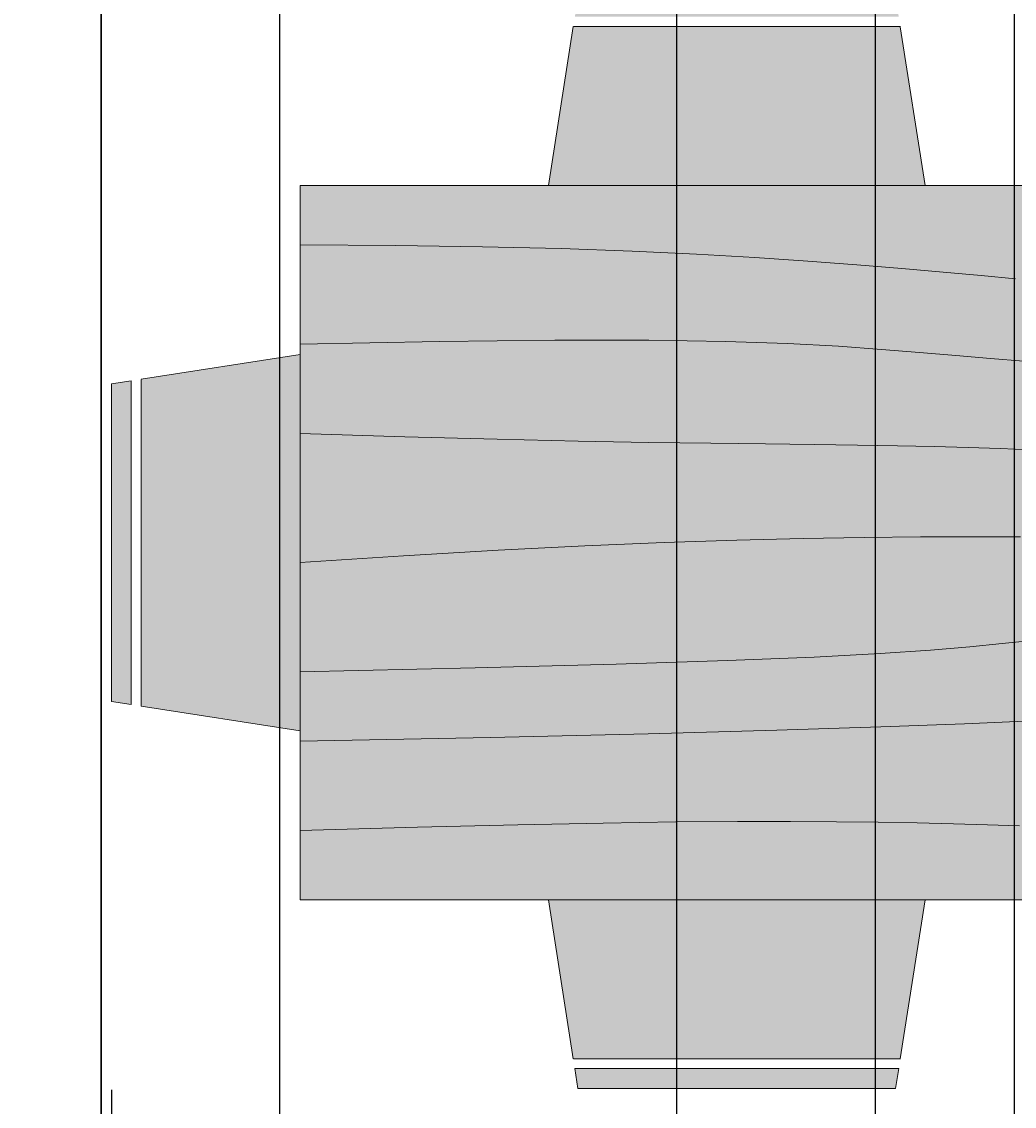
# Model space of a CAD drawing. Units: inches. Extents: x 1567 to 1964, y 1813 to 2447.
# Tile 17 of 28: x 1738 to 1788, y 2172 to 2226. Entities that reach past the tile are written whole.
import ezdxf

# ---------------------------------------------------------------- set-up
doc = ezdxf.new("R2010")
doc.units = ezdxf.units.IN
doc.layers.add('A-ANNO-DIMS', color=2, linetype='Continuous', lineweight=18)
doc.layers.add('A-FURN', color=8, linetype='Continuous', lineweight=18)
doc.layers.add('A-FURN-PATT', color=252, linetype='Continuous', lineweight=13, true_color=0x939598)
doc.styles.get("Standard").update_dxf_attribs({"font": 'arial.ttf'})
doc.dimstyles.get("Standard").update_dxf_attribs({"dimtxt": 0.18, "dimasz": 0.18, "dimexe": 0.18, "dimexo": 0.0625, "dimgap": 0.09, "dimtad": 0, "dimtih": 1, "dimtoh": 1, "dimdec": 4, "dimzin": 0, "dimdsep": 46, "dimtxsty": 'Standard', "dimcen": 0.09, "dimadec": 0, "dimazin": 0, "dimtfac": 1, "dimtdec": 4, "dimtofl": 0, "dimtmove": 0, "dimatfit": 3, "dimfxl": 1, "dimtolj": 1, "dimtzin": 0, "dimarcsym": 0})

# ---------------------------------------------------------------- blocks, each defined once
blk = doc.blocks.new('Dining Set - 36 x 72 in.')
for p, q in [((-22.2343, 26.00059), (-23.4847, 17.99762)), ((-22.2304, 26), (-5.7608, 26)), ((-4.5152, 17.99762), (-5.7655, 25.99926)), ((36, 18), (-36, 18)), ((-36, 18), (-36, -18)), ((-44.0006, 8.23428), (-35.9976, 9.48474)), ((-44, 8.23041), (-44, -8.23915)), ((-45.5, 8), (-44.5004, 8.15617)), ((-45.5, 8), (-45.5, -8)), ((-44.5, -8.15843), (-44.5, 8.15338)), ((-44.4997, -8.15631), (-45.5, -8)), ((-35.9976, -9.48476), (-43.9993, -8.2345)), ((-36, -18), (36, -18)), ((-22.2343, -26.0006), (-23.4847, -17.99762)), ((-4.5152, -17.99762), (-5.7655, -25.99928)), ((-22.2304, -26), (-5.7608, -26)), ((-22, -27.5), (-22.1562, -26.50044)), ((-5.8416, -26.5), (-22.1534, -26.5)), ((-5.8437, -26.49967), (-6, -27.5)), ((-22, -27.5), (-6, -27.5))]:
    blk.add_line(p, q)
for points in [[(-36, 15), (-31.1772, 14.97754), (-26.8079, 14.91406), (-22.8538, 14.81543), (-19.276, 14.6875), (-16.0362, 14.53613), (-13.0957, 14.36718), (-10.4159, 14.18652), (-7.9583, 14), (-5.6904, 13.81315), (-3.6035, 13.63021), (-1.6954, 13.45508), (0.0365, 13.29166)], [(-36, 10), (-28.9766, 10.14274), (-23.1725, 10.20442), (-18.4241, 10.19775), (-14.5677, 10.13541), (-11.4399, 10.03011), (-8.877, 9.89453), (-6.7154, 9.74137), (-4.7917, 9.58333), (-2.9698, 9.43082), (-1.2246, 9.28515), (0.4415, 9.14534)], [(-36, 5.5), (-30.7157, 5.3348), (-26.069, 5.20963), (-21.9946, 5.11767), (-18.4271, 5.05208), (-15.3009, 5.00602), (-12.5508, 4.97265), (-10.1112, 4.94515), (-7.9167, 4.91666), (-5.909, 4.88167), (-4.0586, 4.83984), (-2.3429, 4.79215), (-0.7396, 4.73958), (0.7739, 4.6831)], [(-36, -1), (-30.7915, -0.6591), (-26.0195, -0.38216), (-21.6519, -0.16284), (-17.6563, 0.00521), (-14.0005, 0.12833), (-10.6523, 0.21289), (-7.5796, 0.26522), (-4.75, 0.29166), (-2.134, 0.29793), (0.2878, 0.28711)], [(-36, -6.5), (-27.1843, -6.31267), (-20.084, -6.1263), (-14.469, -5.9419), (-10.1094, -5.76042), (-6.7752, -5.58285), (-4.2363, -5.41016), (-2.2629, -5.24333), (-0.625, -5.08334), (0.8708, -4.93099)], [(-36, -10), (-26.4022, -9.81299), (-18.4675, -9.62891), (-11.9839, -9.45069), (-6.7396, -9.28125), (-2.5226, -9.12354), (0.8789, -8.98047)], [(-36, -14.5), (-30.0881, -14.33513), (-25.0332, -14.21224), (-20.7312, -14.12647), (-17.0781, -14.07292), (-13.97, -14.04671), (-11.3027, -14.04297), (-8.9724, -14.05681), (-6.875, -14.08334), (-4.9224, -14.11833), (-3.0905, -14.16016), (-1.3709, -14.20785), (0.2448, -14.26042)]]:
    blk.add_lwpolyline(points)
blk = doc.blocks.new('*D27')
at = {"layer": 'A-ANNO-DIMS', "color": 0, "lineweight": -2, "transparency": 16777216}
for p, q in [((1742.951, 2172.357), (1742.951, 2158.59)), ((1833.951, 2172.357), (1833.951, 2158.59)), ((1743.131, 2158.77), (1787.5, 2158.77)), ((1833.771, 2158.77), (1789.403, 2158.77))]:
    blk.add_line(p, q, dxfattribs=at)
at = {"layer": 'A-ANNO-DIMS', "color": 0, "transparency": 16777216}
for points in [[(1743.131, 2158.8), (1743.131, 2158.74), (1742.951, 2158.77)], [(1833.771, 2158.8), (1833.771, 2158.74), (1833.951, 2158.77)]]:
    blk.add_solid(points, dxfattribs=at)
at = {"layer": 'Defpoints', "color": 0, "transparency": 16777216}
for p in [(1742.951, 2172.42), (1833.951, 2172.42), (1833.951, 2158.77)]:
    blk.add_point(p, dxfattribs=at)
at = {"layer": 'A-ANNO-DIMS', "color": 0, "transparency": 16777216, "insert": (1788.451, 2158.77), "char_height": 0.18, "attachment_point": 5}
blk.add_mtext('\\A1;DINING SET 91', dxfattribs=at)
blk = doc.blocks.new('*D47')
at = {"layer": 'A-ANNO-DIMS', "color": 0, "lineweight": -2, "transparency": 16777216}
for p, q in [((1742.43, 2331.227), (1742.43, 1813.46)), ((1788.43, 2331.227), (1788.43, 1813.46)), ((1742.61, 1813.64), (1765.207, 1813.64)), ((1788.25, 1813.64), (1765.652, 1813.64))]:
    blk.add_line(p, q, dxfattribs=at)
at = {"layer": 'A-ANNO-DIMS', "color": 0, "transparency": 16777216}
for points in [[(1742.61, 1813.67), (1742.61, 1813.61), (1742.43, 1813.64)], [(1788.25, 1813.67), (1788.25, 1813.61), (1788.43, 1813.64)]]:
    blk.add_solid(points, dxfattribs=at)
at = {"layer": 'Defpoints', "color": 0, "transparency": 16777216}
for p in [(1742.43, 2331.29), (1788.43, 2331.29), (1788.43, 1813.64)]:
    blk.add_point(p, dxfattribs=at)
at = {"layer": 'A-ANNO-DIMS', "color": 0, "transparency": 16777216, "insert": (1765.43, 1813.64), "char_height": 0.18, "attachment_point": 5}
blk.add_mtext('\\A1;46', dxfattribs=at)
blk = doc.blocks.new('*D54')
at = {"layer": 'A-ANNO-DIMS', "color": 0, "lineweight": -2, "transparency": 16777216}
for p, q in [((1711.43, 1964.352), (1711.43, 2447.12)), ((1711.61, 2446.94), (1753.211, 2446.94)), ((1795.25, 2446.94), (1753.648, 2446.94)), ((1795.43, 1964.352), (1795.43, 2447.12))]:
    blk.add_line(p, q, dxfattribs=at)
at = {"layer": 'A-ANNO-DIMS', "color": 0, "transparency": 16777216}
for points in [[(1711.61, 2446.97), (1711.61, 2446.91), (1711.43, 2446.94)], [(1795.25, 2446.97), (1795.25, 2446.91), (1795.43, 2446.94)]]:
    blk.add_solid(points, dxfattribs=at)
at = {"layer": 'Defpoints', "color": 0, "transparency": 16777216}
for p in [(1795.43, 2446.94), (1711.43, 1964.29), (1795.43, 1964.29)]:
    blk.add_point(p, dxfattribs=at)
at = {"layer": 'A-ANNO-DIMS', "color": 0, "transparency": 16777216, "insert": (1753.43, 2446.94), "char_height": 0.18, "attachment_point": 5}
blk.add_mtext('\\A1;84', dxfattribs=at)
blk = doc.blocks.new('*D58')
at = {"layer": 'A-ANNO-DIMS', "color": 0, "lineweight": -2, "transparency": 16777216}
for p, q in [((1742.43, 2127.352), (1742.43, 2447.12)), ((1742.61, 2446.94), (1746.78, 2446.94)), ((1751.25, 2446.94), (1747.079, 2446.94)), ((1751.43, 2127.352), (1751.43, 2447.12))]:
    blk.add_line(p, q, dxfattribs=at)
at = {"layer": 'A-ANNO-DIMS', "color": 0, "transparency": 16777216}
for points in [[(1742.61, 2446.97), (1742.61, 2446.91), (1742.43, 2446.94)], [(1751.25, 2446.97), (1751.25, 2446.91), (1751.43, 2446.94)]]:
    blk.add_solid(points, dxfattribs=at)
at = {"layer": 'Defpoints', "color": 0, "transparency": 16777216}
for p in [(1751.43, 2446.94), (1742.43, 2127.29), (1751.43, 2127.29)]:
    blk.add_point(p, dxfattribs=at)
at = {"layer": 'A-ANNO-DIMS', "color": 0, "transparency": 16777216, "insert": (1746.93, 2446.94), "char_height": 0.18, "attachment_point": 5}
blk.add_mtext('\\A1;9', dxfattribs=at)
blk = doc.blocks.new('*D59')
at = {"layer": 'A-ANNO-DIMS', "color": 0, "lineweight": -2, "transparency": 16777216}
for p, q in [((1751.43, 2127.352), (1751.43, 2447.12)), ((1751.61, 2446.94), (1766.211, 2446.94)), ((1781.25, 2446.94), (1766.648, 2446.94)), ((1781.43, 2127.352), (1781.43, 2447.12))]:
    blk.add_line(p, q, dxfattribs=at)
at = {"layer": 'A-ANNO-DIMS', "color": 0, "transparency": 16777216}
for points in [[(1751.61, 2446.97), (1751.61, 2446.91), (1751.43, 2446.94)], [(1781.25, 2446.97), (1781.25, 2446.91), (1781.43, 2446.94)]]:
    blk.add_solid(points, dxfattribs=at)
at = {"layer": 'Defpoints', "color": 0, "transparency": 16777216}
for p in [(1781.43, 2446.94), (1751.43, 2127.29), (1781.43, 2127.29)]:
    blk.add_point(p, dxfattribs=at)
at = {"layer": 'A-ANNO-DIMS', "color": 0, "transparency": 16777216, "insert": (1766.43, 2446.94), "char_height": 0.18, "attachment_point": 5}
blk.add_mtext('\\A1;30', dxfattribs=at)
blk = doc.blocks.new('*D63')
at = {"layer": 'A-ANNO-DIMS', "color": 0, "lineweight": -2, "transparency": 16777216}
for p, q in [((1735.43, 1988.352), (1735.43, 2447.12)), ((1735.61, 2446.94), (1753.211, 2446.94)), ((1771.25, 2446.94), (1753.648, 2446.94)), ((1771.43, 1988.352), (1771.43, 2447.12))]:
    blk.add_line(p, q, dxfattribs=at)
at = {"layer": 'A-ANNO-DIMS', "color": 0, "transparency": 16777216}
for points in [[(1735.61, 2446.97), (1735.61, 2446.91), (1735.43, 2446.94)], [(1771.25, 2446.97), (1771.25, 2446.91), (1771.43, 2446.94)]]:
    blk.add_solid(points, dxfattribs=at)
at = {"layer": 'Defpoints', "color": 0, "transparency": 16777216}
for p in [(1771.43, 2446.94), (1735.43, 1988.29), (1771.43, 1988.29)]:
    blk.add_point(p, dxfattribs=at)
at = {"layer": 'A-ANNO-DIMS', "color": 0, "transparency": 16777216, "insert": (1753.43, 2446.94), "char_height": 0.18, "attachment_point": 5}
blk.add_mtext('\\A1;36', dxfattribs=at)

msp = doc.modelspace()

# ---------------------------------------------------------------- hatches: boundary and pattern name
at = {"layer": 'A-FURN-PATT'}
h = msp.add_hatch(color=256, dxfattribs=at)
h.dxf.hatch_style = 1
h.paths.add_polyline_path([(1621.2532, 2242.0229), (1643.7811, 2241.7239), (1643.8607, 2247.7234), (1617.863, 2248.0685, 0.1904762), (1616.7481, 2164.0759), (1642.7458, 2163.7308), (1642.8254, 2169.7302), (1620.2975, 2170.0293, -0.1519478)])
h.paths.add_polyline_path([(1673.5306, 2249.6607), (1653.8509, 2249.6607), (1653.8509, 2248.5031, 0.1176471), (1673.5306, 2248.5031)])
h.paths.add_polyline_path([(1706.0889, 2249.6607), (1686.4092, 2249.6607), (1686.4092, 2248.5031, 0.1176471), (1706.0889, 2248.5031)])
h.paths.add_polyline_path([(1782.4511, 2227.4197), (1766.4511, 2227.4197), (1766.2949, 2226.4197), (1782.6074, 2226.4197)])
h.paths.add_polyline_path([(1810.4511, 2227.4197), (1794.4511, 2227.4197), (1794.2949, 2226.4197), (1810.6074, 2226.4197)])
h.paths.add_polyline_path([(1743.9511, 2208.076), (1742.9511, 2207.9197), (1742.9511, 2191.9197), (1743.9511, 2191.7635)])
h.paths.add_polyline_path([(1782.6074, 2173.4197), (1766.2949, 2173.4197), (1766.4511, 2172.4197), (1782.4511, 2172.4197)])
h.paths.add_polyline_path([(1810.6074, 2173.4197), (1794.2949, 2173.4197), (1794.4511, 2172.4197), (1810.4511, 2172.4197)])
h.paths.add_polyline_path([(1861.053, 2006.5071), (1845.8531, 2006.5071), (1861.053, 1991.3071)])
h.paths.add_polyline_path([(1905.853, 1993.7071), (1861.053, 1993.7071), (1861.053, 1991.3071), (1905.853, 1991.3071)])
h.paths.add_polyline_path([(1919.7245, 2257.29, 0.5000001), (1918.7245, 2258.29), (1901.7245, 2258.29, 0.5000001), (1900.7245, 2257.29), (1900.7245, 2253.29, 0.5000001), (1901.7245, 2252.29), (1918.7245, 2252.29, 0.5000001), (1919.7245, 2253.29)])
h.paths.add_polyline_path([(1875.9094, 2391.0204), (1875.9094, 2375.8204), (1891.1093, 2375.8204)], flags=17)
h.paths.add_polyline_path([(1891.1093, 2405.4204), (1831.1094, 2405.4204), (1831.1094, 2391.0204), (1839.1093, 2391.0204), (1839.1093, 2404.2204), (1859.9093, 2404.2204), (1859.9093, 2391.0204), (1862.3093, 2391.0204), (1862.3093, 2404.2204), (1883.1093, 2404.2204), (1883.1093, 2389.0204), (1877.9094, 2389.0204), (1891.1093, 2375.8204)])
h.paths.add_polyline_path([(1682.1402, 2390.0316), (1682.1402, 2374.8316), (1697.3402, 2374.8316)], flags=17)
h.paths.add_polyline_path([(1697.3402, 2404.4316), (1637.3402, 2404.4316), (1637.3402, 2390.0316), (1645.3402, 2390.0316), (1645.3402, 2403.2316), (1666.1402, 2403.2316), (1666.1402, 2390.0316), (1668.5402, 2390.0316), (1668.5402, 2403.2316), (1689.3402, 2403.2316), (1689.3402, 2388.0316), (1684.1402, 2388.0316), (1697.3402, 2374.8316)])
h = msp.add_hatch(color=256, dxfattribs=at)
h.dxf.hatch_style = 1
h.paths.add_polyline_path([(1697.3402, 2374.8316), (1682.1402, 2374.8316), (1682.1402, 2387.6316), (1637.3402, 2387.6316), (1637.3402, 2324.4315), (1697.3402, 2324.4315)])
h.paths.add_polyline_path([(1891.1093, 2375.8204), (1875.9094, 2375.8204), (1875.9094, 2388.6204), (1831.1094, 2388.6204), (1831.1094, 2325.4204), (1891.1093, 2325.4204)])
h.paths.add_polyline_path([(1702.5611, 2206.8057), (1702.5611, 2210.8057), (1699.7395, 2209.9436), (1697.013, 2209.2403), (1694.3857, 2208.6763), (1691.8615, 2208.2326), (1689.4443, 2207.8896), (1687.1381, 2207.6282), (1684.9469, 2207.4289), (1682.8747, 2207.2725), (1680.9233, 2207.1425), (1679.0865, 2207.0339), (1677.3558, 2206.9445), (1675.7229, 2206.8719), (1674.1794, 2206.8141), (1672.7169, 2206.7688), (1671.327, 2206.7339), (1670.0014, 2206.707), (1668.7314, 2206.6866), (1667.5072, 2206.6732), (1666.3188, 2206.668), (1665.1561, 2206.6722), (1664.009, 2206.6869), (1662.8675, 2206.7133), (1661.7215, 2206.7525), (1660.5611, 2206.8057), (1660.5611, 2202.8057), (1661.9932, 2202.9556), (1663.3314, 2203.0744), (1664.5899, 2203.1671), (1665.7831, 2203.2385), (1666.9254, 2203.2935), (1668.0311, 2203.3368), (1669.1145, 2203.3734), (1670.1902, 2203.4081), (1671.2724, 2203.4451), (1672.3759, 2203.4866), (1673.5155, 2203.534), (1674.706, 2203.5887), (1675.9621, 2203.6523), (1677.2986, 2203.7262), (1678.7304, 2203.8118), (1680.2722, 2203.9108), (1681.947, 2204.0272), (1683.8108, 2204.1769), (1685.9279, 2204.3782), (1688.3626, 2204.6496), (1691.179, 2205.0096), (1694.4413, 2205.4767), (1698.214, 2206.0692)])
h.paths.add_polyline_path([(1702.5611, 2218.8057), (1701.9821, 2217.9383), (1701.3316, 2217.191), (1700.6091, 2216.5515), (1699.8141, 2216.0071), (1698.946, 2215.5454), (1698.0041, 2215.1536), (1696.9879, 2214.8194), (1695.8969, 2214.5301), (1694.7328, 2214.2753), (1693.5072, 2214.0522), (1692.2339, 2213.8602), (1690.9266, 2213.6989), (1689.5994, 2213.5675), (1688.266, 2213.4654), (1686.9402, 2213.392), (1685.636, 2213.3467), (1684.3619, 2213.3287), (1683.1053, 2213.3361), (1681.8482, 2213.3668), (1680.5727, 2213.4187), (1679.2608, 2213.4898), (1677.8948, 2213.5779), (1676.4565, 2213.6811), (1674.9282, 2213.7971), (1673.2982, 2213.9236), (1671.5804, 2214.0573), (1669.795, 2214.1945), (1667.9622, 2214.3316), (1666.1022, 2214.4649), (1664.2352, 2214.5908), (1662.3814, 2214.7056), (1660.5611, 2214.8057), (1660.5611, 2206.8057), (1661.7215, 2206.7525), (1662.8675, 2206.7133), (1664.009, 2206.6869), (1665.1561, 2206.6722), (1666.3188, 2206.668), (1667.5072, 2206.6732), (1668.7314, 2206.6866), (1670.0014, 2206.707), (1671.327, 2206.7339), (1672.7169, 2206.7688), (1674.1794, 2206.8141), (1675.7229, 2206.8719), (1677.3558, 2206.9445), (1679.0865, 2207.0339), (1680.9233, 2207.1425), (1682.8747, 2207.2725), (1684.9469, 2207.4289), (1687.1381, 2207.6282), (1689.4443, 2207.8896), (1691.8615, 2208.2326), (1694.3857, 2208.6763), (1697.013, 2209.2403), (1699.7395, 2209.9436), (1702.5611, 2210.8057)])
h.paths.add_polyline_path([(1700.6091, 2216.5515), (1701.3316, 2217.191), (1701.9821, 2217.9383), (1702.5611, 2218.8057), (1702.5611, 2222.8057), (1689.452, 2222.8057), (1689.0171, 2222.4556), (1688.4521, 2222.0354), (1687.7806, 2221.5662), (1687.0235, 2221.067), (1686.2019, 2220.5566), (1685.3367, 2220.0541), (1684.4491, 2219.5785), (1683.56, 2219.1486), (1682.6867, 2218.7795), (1681.8312, 2218.4692), (1680.9918, 2218.212), (1680.1667, 2218.0019), (1679.3541, 2217.833), (1678.5524, 2217.6995), (1677.7597, 2217.5954), (1676.9744, 2217.5149), (1676.1942, 2217.4531), (1675.4146, 2217.4093), (1674.6309, 2217.384), (1673.8381, 2217.3774), (1673.0313, 2217.39), (1672.2056, 2217.4221), (1671.3562, 2217.4741), (1670.4782, 2217.5463), (1669.5642, 2217.639), (1668.5968, 2217.7516), (1667.5562, 2217.8833), (1666.4226, 2218.0336), (1665.1761, 2218.2017), (1663.7969, 2218.3869), (1662.2651, 2218.5885), (1660.5611, 2218.8057), (1660.5611, 2214.8057), (1662.3814, 2214.7056), (1664.2352, 2214.5908), (1666.1022, 2214.4649), (1667.9622, 2214.3316), (1669.795, 2214.1945), (1671.5804, 2214.0573), (1673.2982, 2213.9236), (1674.9282, 2213.7971), (1676.4565, 2213.6811), (1677.8948, 2213.5779), (1679.2608, 2213.4898), (1680.5727, 2213.4187), (1681.8482, 2213.3668), (1683.1053, 2213.3361), (1684.3619, 2213.3287), (1685.636, 2213.3467), (1686.9402, 2213.392), (1688.266, 2213.4654), (1689.5994, 2213.5675), (1690.9266, 2213.6989), (1692.2339, 2213.8602), (1693.5072, 2214.0522), (1694.7328, 2214.2753), (1695.8969, 2214.5301), (1696.9879, 2214.8194), (1698.0041, 2215.1536), (1698.946, 2215.5454), (1699.8141, 2216.0071)])
h.paths.add_polyline_path([(1687.0235, 2221.067), (1687.7806, 2221.5662), (1688.4521, 2222.0354), (1689.0171, 2222.4556), (1689.452, 2222.8057), (1660.5611, 2222.8057), (1660.5611, 2218.8057), (1662.2651, 2218.5885), (1663.7969, 2218.3869), (1665.1761, 2218.2017), (1666.4226, 2218.0336), (1667.5562, 2217.8833), (1668.5968, 2217.7516), (1669.5642, 2217.639), (1670.4782, 2217.5463), (1671.3562, 2217.4741), (1672.2056, 2217.4221), (1673.0313, 2217.39), (1673.8381, 2217.3774), (1674.6309, 2217.384), (1675.4146, 2217.4093), (1676.1942, 2217.4531), (1676.9744, 2217.5149), (1677.7597, 2217.5954), (1678.5524, 2217.6995), (1679.3541, 2217.833), (1680.1667, 2218.0019), (1680.9918, 2218.212), (1681.8312, 2218.4692), (1682.6867, 2218.7795), (1683.56, 2219.1486), (1684.4491, 2219.5785), (1685.3367, 2220.0541), (1686.2019, 2220.5566)], flags=17)
h.paths.add_polyline_path([(1702.5611, 2198.8057), (1698.9289, 2199.2412), (1695.8472, 2199.5774), (1693.2166, 2199.8257), (1690.9377, 2199.9973), (1688.9111, 2200.1033), (1687.0375, 2200.155), (1685.2174, 2200.1637), (1683.3514, 2200.1406), (1681.3514, 2200.0941), (1679.1736, 2200.0225), (1676.7858, 2199.921), (1674.1554, 2199.7852), (1671.2502, 2199.6103), (1668.0377, 2199.3919), (1664.4854, 2199.1252), (1660.5611, 2198.8057), (1660.5611, 2194.8057), (1662.2697, 2194.9771), (1663.9673, 2195.0999), (1665.6339, 2195.1809), (1667.2495, 2195.227), (1668.7941, 2195.2449), (1670.2478, 2195.2414), (1671.5906, 2195.2233), (1672.8026, 2195.1974), (1673.8739, 2195.1689), (1674.8359, 2195.1364), (1675.7302, 2195.0967), (1676.5982, 2195.0469), (1677.4817, 2194.9838), (1678.422, 2194.9043), (1679.4609, 2194.8055), (1680.6397, 2194.6842), (1682.005, 2194.5341), (1683.6223, 2194.335), (1685.562, 2194.0637), (1687.8945, 2193.6967), (1690.6902, 2193.2108), (1694.0196, 2192.5826), (1697.9531, 2191.7887), (1702.5611, 2190.8057)])
h.paths.add_polyline_path([(1702.5611, 2206.8057), (1698.214, 2206.0692), (1694.4413, 2205.4767), (1691.179, 2205.0096), (1688.3626, 2204.6496), (1685.9279, 2204.3782), (1683.8108, 2204.1769), (1681.947, 2204.0272), (1680.2722, 2203.9108), (1678.7304, 2203.8118), (1677.2986, 2203.7262), (1675.9621, 2203.6523), (1674.706, 2203.5887), (1673.5155, 2203.534), (1672.3759, 2203.4866), (1671.2724, 2203.4451), (1670.1902, 2203.4081), (1669.1145, 2203.3734), (1668.0311, 2203.3368), (1666.9254, 2203.2935), (1665.7831, 2203.2385), (1664.5899, 2203.1671), (1663.3314, 2203.0744), (1661.9932, 2202.9556), (1660.5611, 2202.8057), (1660.5611, 2198.8057), (1664.4854, 2199.1252), (1668.0377, 2199.3919), (1671.2502, 2199.6103), (1674.1554, 2199.7852), (1676.7858, 2199.921), (1679.1736, 2200.0225), (1681.3514, 2200.0941), (1683.3514, 2200.1406), (1685.2174, 2200.1637), (1687.0375, 2200.155), (1688.9111, 2200.1033), (1690.9377, 2199.9973), (1693.2166, 2199.8257), (1695.8472, 2199.5774), (1698.9289, 2199.2412), (1702.5611, 2198.8057)])
h.paths.add_polyline_path([(1702.5611, 2190.8057), (1697.9531, 2191.7887), (1694.0196, 2192.5826), (1690.6902, 2193.2108), (1687.8945, 2193.6967), (1685.562, 2194.0637), (1683.6223, 2194.335), (1682.005, 2194.5341), (1680.6397, 2194.6842), (1679.4609, 2194.8055), (1678.422, 2194.9043), (1677.4817, 2194.9838), (1676.5982, 2195.0469), (1675.7302, 2195.0967), (1674.8359, 2195.1364), (1673.8739, 2195.1689), (1672.8026, 2195.1974), (1671.5906, 2195.2233), (1670.2478, 2195.2414), (1668.7941, 2195.2449), (1667.2495, 2195.227), (1665.6339, 2195.1809), (1663.9673, 2195.0999), (1662.2697, 2194.9771), (1660.5611, 2194.8057), (1660.5611, 2190.8057), (1665.9637, 2190.2699), (1670.5105, 2189.7867), (1674.3035, 2189.3504), (1677.4445, 2188.9552), (1680.0354, 2188.5951), (1682.1782, 2188.2644), (1683.9747, 2187.9571), (1685.5268, 2187.6675), (1686.9225, 2187.3901), (1688.1943, 2187.1216), (1689.3606, 2186.859), (1690.4399, 2186.5993), (1691.4508, 2186.3396), (1692.4118, 2186.0769), (1693.3413, 2185.8084), (1694.2579, 2185.531), (1695.1786, 2185.2422), (1696.1142, 2184.9406), (1697.0739, 2184.6252), (1698.0671, 2184.2949), (1699.1032, 2183.9489), (1700.1913, 2183.586), (1701.3408, 2183.2053), (1702.5611, 2182.8057)])
h.paths.add_polyline_path([(1702.5611, 2182.8057), (1701.3408, 2183.2053), (1700.1913, 2183.586), (1699.1032, 2183.9489), (1698.0671, 2184.2949), (1697.0739, 2184.6252), (1696.1142, 2184.9406), (1695.1786, 2185.2422), (1694.2579, 2185.531), (1693.3413, 2185.8084), (1692.4118, 2186.0769), (1691.4508, 2186.3396), (1690.4399, 2186.5993), (1689.3606, 2186.859), (1688.1943, 2187.1216), (1686.9225, 2187.3901), (1685.5268, 2187.6675), (1683.9747, 2187.9571), (1682.1782, 2188.2644), (1680.0354, 2188.5951), (1677.4445, 2188.9552), (1674.3035, 2189.3504), (1670.5105, 2189.7867), (1665.9637, 2190.2699), (1660.5611, 2190.8057), (1660.5611, 2186.8057), (1663.5709, 2186.52), (1666.0965, 2186.2414), (1668.1979, 2185.9698), (1669.9351, 2185.7048), (1671.3681, 2185.446), (1672.5568, 2185.1931), (1673.5613, 2184.9458), (1674.4415, 2184.7037), (1675.2485, 2184.4664), (1675.9976, 2184.2328), (1677.0295, 2183.8907), (1678.2492, 2183.4332), (1679.354, 2182.9669), (1680.4123, 2182.4724), (1681.3757, 2181.9718), (1682.2435, 2181.4594), (1683.1864, 2180.8057), (1702.5611, 2180.8057)])
h.paths.add_polyline_path([(1677.3469, 2183.7716), (1676.6949, 2184.0016), (1675.9976, 2184.2328), (1675.2485, 2184.4664), (1674.4415, 2184.7037), (1673.5613, 2184.9458), (1672.5568, 2185.1931), (1671.3681, 2185.446), (1669.9351, 2185.7048), (1668.1979, 2185.9698), (1666.0965, 2186.2414), (1663.5709, 2186.52), (1660.5611, 2186.8057), (1660.5611, 2180.8057), (1683.1506, 2180.8057), (1682.802, 2181.0722), (1682.4264, 2181.3326), (1682.0201, 2181.5913), (1681.586, 2181.8476), (1681.1268, 2182.1011), (1680.6453, 2182.3513), (1680.1443, 2182.5976), (1679.6266, 2182.8395), (1679.0933, 2183.0769), (1678.5398, 2183.3105), (1677.9598, 2183.5417)], flags=17)
h.paths.add_polyline_path([(1824.4511, 2199.9016), (1824.089, 2199.9302), (1824.0595, 2199.9372), (1824.0397, 2199.9406), (1823.5413, 2200.0576), (1823.4095, 2200.0864), (1823.0664, 2200.1559), (1822.6419, 2200.2361), (1822.1519, 2200.3222), (1821.6126, 2200.4093), (1821.0401, 2200.4925), (1820.4505, 2200.5669), (1819.8599, 2200.6276), (1819.2845, 2200.6697), (1818.7366, 2200.6896), (1818.2141, 2200.688), (1817.7112, 2200.6668), (1817.222, 2200.6281), (1816.7405, 2200.5737), (1816.261, 2200.5057), (1815.7776, 2200.4259), (1815.2845, 2200.3364), (1814.3007, 2200.149), (1813.3315, 2199.9765), (1812.406, 2199.8514), (1811.6868, 2199.7739), (1810.8992, 2199.7121), (1810.0345, 2199.6697), (1809.0854, 2199.6497), (1808.0514, 2199.6502), (1806.9334, 2199.6683), (1805.7324, 2199.701), (1804.4493, 2199.7454), (1803.0852, 2199.7986), (1801.641, 2199.8577), (1800.1178, 2199.9197), (1798.5134, 2199.9818), (1796.8144, 2200.0415), (1795.004, 2200.0962), (1793.0657, 2200.1437), (1790.9828, 2200.1814), (1788.7389, 2200.2068), (1786.3171, 2200.2177), (1783.7011, 2200.2114), (1780.8715, 2200.185), (1777.7988, 2200.1326), (1774.4506, 2200.0481), (1770.7948, 2199.9249), (1766.7992, 2199.7569), (1762.4316, 2199.5376), (1757.6596, 2199.2606), (1752.4511, 2198.9197), (1752.4511, 2193.4197), (1761.2668, 2193.6071), (1768.3671, 2193.7934), (1773.9821, 2193.9778), (1778.3417, 2194.1593), (1781.6759, 2194.3369), (1784.2148, 2194.5096), (1786.1882, 2194.6764), (1787.8261, 2194.8364), (1789.3219, 2194.9887), (1790.7226, 2195.1333), (1792.0383, 2195.27), (1793.2792, 2195.3989), (1794.4557, 2195.52), (1795.5781, 2195.6333), (1796.6564, 2195.7387), (1797.7011, 2195.8364), (1798.7216, 2195.9259), (1799.7245, 2196.0057), (1800.7158, 2196.0737), (1801.7011, 2196.1281), (1802.6865, 2196.1668), (1803.6777, 2196.188), (1804.6806, 2196.1896), (1805.7011, 2196.1697), (1806.7423, 2196.1273), (1807.7962, 2196.0643), (1808.852, 2195.9837), (1809.899, 2195.8885), (1810.9265, 2195.7815), (1811.9238, 2195.6658), (1812.88, 2195.5442), (1813.7845, 2195.4197), (1814.6296, 2195.2948), (1815.4205, 2195.1704), (1816.1656, 2195.0469), (1816.873, 2194.9249), (1817.5511, 2194.8049), (1818.2083, 2194.6873), (1818.8527, 2194.5726), (1819.4928, 2194.4614), (1820.1348, 2194.3554), (1820.7773, 2194.2615), (1821.4169, 2194.1882), (1822.0501, 2194.1437), (1822.6735, 2194.1363), (1823.2838, 2194.1743), (1823.8775, 2194.266), (1824.4511, 2194.4197)])
h.paths.add_polyline_path([(1821.4716, 2190.5098), (1820.4303, 2190.5708), (1819.3811, 2190.6415), (1818.3339, 2190.7186), (1817.2985, 2190.7986), (1816.2845, 2190.8781), (1815.2976, 2190.9542), (1814.3274, 2191.0259), (1813.3592, 2191.0927), (1812.3782, 2191.1541), (1811.3699, 2191.2097), (1810.3196, 2191.2589), (1809.2127, 2191.3013), (1808.0345, 2191.3364), (1806.7708, 2191.3634), (1805.4094, 2191.3807), (1803.9387, 2191.3862), (1802.3469, 2191.3781), (1800.6223, 2191.3543), (1798.7532, 2191.313), (1796.7278, 2191.2521), (1794.5344, 2191.1697), (1792.128, 2191.0648), (1789.33, 2190.9393), (1785.9285, 2190.7962), (1781.7115, 2190.6385), (1776.4672, 2190.469), (1769.9836, 2190.2908), (1762.0489, 2190.1067), (1752.4511, 2189.9197), (1752.4511, 2185.4197), (1758.363, 2185.5846), (1763.4179, 2185.7075), (1767.7199, 2185.7933), (1771.373, 2185.8468), (1774.4811, 2185.873), (1777.1484, 2185.8768), (1779.4787, 2185.8629), (1781.5761, 2185.8364), (1783.5287, 2185.8014), (1785.3606, 2185.7596), (1787.0802, 2185.7119), (1788.6959, 2185.6593), (1790.2158, 2185.6028), (1791.6484, 2185.5434), (1793.0018, 2185.4821), (1794.2844, 2185.4197), (1795.5065, 2185.3576), (1796.6861, 2185.298), (1797.8433, 2185.2432), (1798.998, 2185.1958), (1800.1703, 2185.1581), (1801.3801, 2185.1326), (1802.6476, 2185.1218), (1803.9928, 2185.1281), (1805.4444, 2185.1555), (1807.0663, 2185.2147), (1808.9315, 2185.3178), (1811.1126, 2185.477), (1813.6823, 2185.7046), (1816.7135, 2186.0128), (1820.2788, 2186.4138), (1824.4511, 2186.9197), (1824.4511, 2190.4197), (1823.4918, 2190.4309), (1822.4954, 2190.4621)])
h.paths.add_polyline_path([(1797.3762, 2216.0584), (1797.6199, 2216.2267), (1797.9558, 2216.3355), (1798.3017, 2216.3703), (1798.5761, 2216.3781), (1798.8974, 2216.3703), (1799.2714, 2216.3468), (1799.704, 2216.3078), (1800.2011, 2216.2531), (1800.7695, 2216.1829), (1801.4205, 2216.0981), (1802.1662, 2215.9996), (1803.0188, 2215.8885), (1803.9906, 2215.7656), (1805.0937, 2215.632), (1806.3404, 2215.4886), (1807.7428, 2215.3364), (1809.3101, 2215.1764), (1811.039, 2215.0096), (1812.9232, 2214.8369), (1814.9563, 2214.6593), (1817.132, 2214.4778), (1819.444, 2214.2934), (1821.8858, 2214.1071), (1824.4511, 2213.9197), (1824.4511, 2217.9197), (1752.4511, 2217.9197), (1752.4511, 2214.9197), (1757.2739, 2214.8973), (1761.6432, 2214.8338), (1765.5973, 2214.7352), (1769.1751, 2214.6072), (1772.4149, 2214.4559), (1775.3554, 2214.2869), (1778.0352, 2214.1063), (1780.4928, 2213.9197), (1782.7607, 2213.7329), (1784.8476, 2213.5499), (1786.7557, 2213.3748), (1788.4876, 2213.2114), (1790.0456, 2213.0636), (1791.4322, 2212.9354), (1792.6499, 2212.8305), (1793.7011, 2212.7531), (1794.5904, 2212.7059), (1795.3313, 2212.688), (1795.9394, 2212.6974), (1796.4303, 2212.7322), (1796.8196, 2212.7905), (1797.123, 2212.8703), (1797.356, 2212.9695), (1797.5344, 2213.0864), (1797.6716, 2213.2187), (1797.7727, 2213.3637), (1797.8406, 2213.5185), (1797.8782, 2213.6801), (1797.8884, 2213.8457), (1797.8743, 2214.0122), (1797.8386, 2214.1767), (1797.7844, 2214.3364), (1797.7149, 2214.4889), (1797.6347, 2214.6346), (1797.5486, 2214.7744), (1797.3327, 2215.109), (1797.178, 2215.4303), (1797.1896, 2215.7939)])
h.paths.add_polyline_path([(1804.7872, 2210.6789), (1804.546, 2211.022), (1804.3512, 2211.3917), (1804.2466, 2211.7546), (1804.2574, 2212.0998), (1804.4058, 2212.4178), (1804.7068, 2212.7007), (1805.1359, 2212.9124), (1805.5279, 2212.9926), (1805.8136, 2213.0154), (1806.1178, 2213.0031), (1806.4405, 2212.9529), (1806.7929, 2212.867), (1807.1893, 2212.7489), (1807.6438, 2212.602), (1808.1706, 2212.4297), (1808.7838, 2212.2355), (1809.4976, 2212.0227), (1810.3261, 2211.7947), (1811.2868, 2211.5533), (1812.4101, 2211.2928), (1813.7297, 2211.0059), (1815.2793, 2210.6854), (1817.0925, 2210.3238), (1819.2031, 2209.9139), (1821.6447, 2209.4483), (1824.4511, 2208.9197), (1824.4511, 2213.9197), (1821.8858, 2214.1071), (1819.444, 2214.2934), (1817.132, 2214.4778), (1814.9563, 2214.6593), (1812.9232, 2214.8369), (1811.039, 2215.0096), (1809.3101, 2215.1764), (1807.7428, 2215.3364), (1806.3404, 2215.4886), (1805.0937, 2215.632), (1803.9906, 2215.7656), (1803.0188, 2215.8885), (1802.1662, 2215.9996), (1801.4205, 2216.0981), (1800.7695, 2216.1829), (1800.2011, 2216.2531), (1799.704, 2216.3078), (1799.2714, 2216.3468), (1798.8974, 2216.3703), (1798.5761, 2216.3781), (1798.3017, 2216.3703), (1798.0683, 2216.3468), (1797.87, 2216.3078), (1797.7011, 2216.2531), (1797.5566, 2216.1831), (1797.4355, 2216.0994), (1797.3378, 2216.004), (1797.2636, 2215.8989), (1797.2128, 2215.7859), (1797.1855, 2215.6671), (1797.1816, 2215.5444), (1797.2011, 2215.4197), (1797.2433, 2215.2946), (1797.304, 2215.1684), (1797.3783, 2215.0403), (1797.4615, 2214.9093), (1797.6718, 2214.5836), (1797.8218, 2214.2545), (1797.8933, 2213.9247), (1797.8728, 2213.5918), (1797.7366, 2213.2814), (1797.4586, 2213.0132), (1797.123, 2212.8703), (1796.8196, 2212.7905), (1796.4303, 2212.7322), (1795.9394, 2212.6974), (1795.3313, 2212.688), (1794.5904, 2212.7059), (1793.7011, 2212.7531), (1792.6499, 2212.8305), (1791.4322, 2212.9354), (1790.0456, 2213.0636), (1788.4876, 2213.2114), (1786.7557, 2213.3748), (1784.8476, 2213.5499), (1782.7607, 2213.7329), (1780.4928, 2213.9197), (1778.0352, 2214.1063), (1775.3554, 2214.2869), (1772.4149, 2214.4559), (1769.1751, 2214.6072), (1765.5973, 2214.7352), (1761.6432, 2214.8338), (1757.2739, 2214.8973), (1752.4511, 2214.9197), (1752.4511, 2209.9197), (1759.4745, 2210.0625), (1765.2786, 2210.1242), (1770.027, 2210.1175), (1773.8834, 2210.0551), (1777.0112, 2209.9498), (1779.5741, 2209.8143), (1781.7357, 2209.6611), (1783.6594, 2209.5031), (1785.4813, 2209.3506), (1787.2265, 2209.2049), (1788.8926, 2209.0651), (1790.4771, 2208.9301), (1791.9777, 2208.7991), (1793.3919, 2208.671), (1794.7171, 2208.5449), (1795.9511, 2208.4197), (1797.0922, 2208.2952), (1798.1425, 2208.1736), (1799.1049, 2208.0579), (1799.9823, 2207.951), (1800.7778, 2207.8558), (1801.4941, 2207.7752), (1802.1342, 2207.7122), (1802.7011, 2207.6697), (1803.1982, 2207.65), (1803.6308, 2207.6528), (1804.0048, 2207.6771), (1804.3261, 2207.7218), (1804.6005, 2207.7861), (1804.8339, 2207.869), (1805.0322, 2207.9694), (1805.2011, 2208.0864), (1805.3455, 2208.2189), (1805.4654, 2208.365), (1805.56, 2208.5229), (1805.6282, 2208.6906), (1805.6691, 2208.866), (1805.6816, 2209.0473), (1805.6648, 2209.2326), (1805.6178, 2209.4197), (1805.5406, 2209.6072), (1805.4381, 2209.7947), (1805.316, 2209.9822), (1805.1803, 2210.1697), (1805.0367, 2210.3572)])
h.paths.add_polyline_path([(1801.4941, 2207.7752), (1800.7778, 2207.8558), (1799.9823, 2207.951), (1799.1049, 2208.0579), (1798.1425, 2208.1736), (1797.0922, 2208.2952), (1795.9511, 2208.4197), (1794.7171, 2208.5449), (1793.3919, 2208.671), (1791.9777, 2208.7991), (1790.4771, 2208.9301), (1788.8926, 2209.0651), (1787.2265, 2209.2049), (1785.4813, 2209.3506), (1783.6594, 2209.5031), (1781.7357, 2209.6611), (1779.5741, 2209.8143), (1777.0112, 2209.9498), (1773.8834, 2210.0551), (1770.027, 2210.1175), (1765.2786, 2210.1242), (1759.4745, 2210.0625), (1752.4511, 2209.9197), (1752.4511, 2205.4197), (1757.7354, 2205.2545), (1762.3821, 2205.1294), (1766.4565, 2205.0374), (1770.024, 2204.9718), (1773.1502, 2204.9258), (1775.9003, 2204.8924), (1778.3399, 2204.8649), (1780.5344, 2204.8364), (1782.5421, 2204.8014), (1784.3925, 2204.7596), (1786.1082, 2204.7119), (1787.7115, 2204.6593), (1789.225, 2204.6028), (1790.6711, 2204.5434), (1792.0724, 2204.4821), (1793.4511, 2204.4197), (1794.8241, 2204.3576), (1796.1855, 2204.2973), (1797.5234, 2204.241), (1798.8261, 2204.1906), (1800.082, 2204.1479), (1801.2792, 2204.115), (1802.4062, 2204.0939), (1803.4511, 2204.0864), (1804.4051, 2204.0942), (1805.2701, 2204.1176), (1806.0512, 2204.1567), (1806.7532, 2204.2114), (1807.381, 2204.2817), (1807.9394, 2204.3676), (1808.4334, 2204.4692), (1808.8678, 2204.5864), (1809.248, 2204.7187), (1809.5813, 2204.8637), (1809.8756, 2205.0185), (1810.1386, 2205.1801), (1810.3782, 2205.3457), (1810.6022, 2205.5122), (1810.9725, 2205.7941), (1811.3803, 2206.072), (1811.739, 2206.2612), (1812.0032, 2206.3781), (1812.2869, 2206.4793), (1812.5931, 2206.563), (1812.9246, 2206.6271), (1813.2845, 2206.6697), (1813.6746, 2206.6894), (1814.0931, 2206.6867), (1814.5369, 2206.6624), (1815.0032, 2206.6176), (1815.489, 2206.5534), (1815.9915, 2206.4705), (1816.5076, 2206.3701), (1817.0345, 2206.2531), (1817.5753, 2206.1196), (1818.1582, 2205.9666), (1818.8172, 2205.7902), (1819.5865, 2205.5864), (1820.5004, 2205.3514), (1821.5931, 2205.0812), (1822.8986, 2204.7719), (1824.4511, 2204.4197), (1824.4511, 2208.9197), (1821.6447, 2209.4483), (1819.2031, 2209.9139), (1817.0925, 2210.3238), (1815.2793, 2210.6854), (1813.7297, 2211.0059), (1812.4101, 2211.2928), (1811.2868, 2211.5533), (1810.3261, 2211.7947), (1809.4976, 2212.0227), (1808.7838, 2212.2355), (1808.1706, 2212.4297), (1807.6438, 2212.602), (1807.1893, 2212.7489), (1806.7929, 2212.867), (1806.4405, 2212.9529), (1806.1178, 2213.0031), (1805.8136, 2213.0154), (1805.5279, 2212.9926), (1805.2638, 2212.9386), (1805.024, 2212.8572), (1804.8116, 2212.7524), (1804.6295, 2212.6281), (1804.4806, 2212.4881), (1804.3678, 2212.3364), (1804.2931, 2212.1764), (1804.2545, 2212.0096), (1804.2491, 2211.8369), (1804.274, 2211.6593), (1804.3263, 2211.4778), (1804.4029, 2211.2934), (1804.5011, 2211.1071), (1804.6178, 2210.9197), (1804.7496, 2210.7322), (1804.8912, 2210.5447), (1805.154, 2210.2061), (1805.3962, 2209.8715), (1805.5964, 2209.5053), (1805.688, 2209.1402), (1805.6629, 2208.7758), (1805.5257, 2208.4385), (1805.2839, 2208.1437), (1804.9434, 2207.9078), (1804.6005, 2207.7861), (1804.3261, 2207.7218), (1804.0048, 2207.6771), (1803.6308, 2207.6528), (1803.1982, 2207.65), (1802.7011, 2207.6697), (1802.1342, 2207.7122)])
h.paths.add_polyline_path([(1824.4511, 2204.4197), (1822.8986, 2204.7719), (1821.5931, 2205.0812), (1820.5004, 2205.3514), (1819.5865, 2205.5864), (1818.8172, 2205.7902), (1818.1582, 2205.9666), (1817.5753, 2206.1196), (1817.0345, 2206.2531), (1816.5076, 2206.3701), (1815.9915, 2206.4705), (1815.489, 2206.5534), (1815.0032, 2206.6176), (1814.5369, 2206.6624), (1814.0931, 2206.6867), (1813.6746, 2206.6894), (1813.2845, 2206.6697), (1812.9246, 2206.6271), (1812.5931, 2206.563), (1812.2869, 2206.4793), (1812.0032, 2206.3781), (1811.739, 2206.2612), (1811.4915, 2206.1307), (1811.2576, 2205.9884), (1811.0345, 2205.8364), (1810.8183, 2205.6767), (1810.4357, 2205.3854), (1810.1386, 2205.1801), (1809.8756, 2205.0185), (1809.5813, 2204.8637), (1809.248, 2204.7187), (1808.8678, 2204.5864), (1808.4334, 2204.4692), (1807.9394, 2204.3676), (1807.381, 2204.2817), (1806.7532, 2204.2114), (1806.0512, 2204.1567), (1805.2701, 2204.1176), (1804.4051, 2204.0942), (1803.4511, 2204.0864), (1802.4062, 2204.0939), (1801.2792, 2204.115), (1800.082, 2204.1479), (1798.8261, 2204.1906), (1797.5234, 2204.241), (1796.1855, 2204.2973), (1794.8241, 2204.3576), (1793.4511, 2204.4197), (1792.0724, 2204.4821), (1790.6711, 2204.5434), (1789.225, 2204.6028), (1787.7115, 2204.6593), (1786.1082, 2204.7119), (1784.3925, 2204.7596), (1782.5421, 2204.8014), (1780.5344, 2204.8364), (1778.3399, 2204.8649), (1775.9003, 2204.8924), (1773.1502, 2204.9258), (1770.024, 2204.9718), (1766.4565, 2205.0374), (1762.3821, 2205.1294), (1757.7354, 2205.2545), (1752.4511, 2205.4197), (1752.4511, 2198.9197), (1757.6596, 2199.2606), (1762.4316, 2199.5376), (1766.7992, 2199.7569), (1770.7948, 2199.9249), (1774.4506, 2200.0481), (1777.7988, 2200.1326), (1780.8715, 2200.185), (1783.7011, 2200.2114), (1786.3171, 2200.2177), (1788.7389, 2200.2068), (1790.9828, 2200.1814), (1793.0657, 2200.1437), (1795.004, 2200.0962), (1796.8144, 2200.0415), (1798.5134, 2199.9818), (1800.1178, 2199.9197), (1801.641, 2199.8577), (1803.0852, 2199.7986), (1804.4493, 2199.7454), (1805.7324, 2199.701), (1806.9334, 2199.6683), (1808.0514, 2199.6502), (1809.0854, 2199.6497), (1810.0345, 2199.6697), (1810.8992, 2199.7121), (1811.6868, 2199.7739), (1812.406, 2199.8514), (1813.0657, 2199.9406), (1813.6746, 2200.0376), (1814.2415, 2200.1385), (1814.7752, 2200.2394), (1815.2845, 2200.3364), (1815.7776, 2200.4259), (1816.261, 2200.5057), (1816.7405, 2200.5737), (1817.222, 2200.6281), (1817.7112, 2200.6668), (1818.2141, 2200.688), (1818.7366, 2200.6896), (1819.2845, 2200.6697), (1819.8599, 2200.6276), (1820.4505, 2200.5669), (1821.0401, 2200.4925), (1821.6126, 2200.4093), (1822.1519, 2200.3222), (1822.6419, 2200.2361), (1823.0664, 2200.1559), (1823.5408, 2200.0598), (1824.0595, 2199.9372), (1824.1105, 2199.9285), (1824.1888, 2199.9223), (1824.2953, 2199.9201), (1824.4511, 2199.9197)])
h.paths.add_polyline_path([(1795.4295, 2021.5492), (1771.4295, 2021.5492), (1771.4295, 1988.29), (1735.4295, 1988.29), (1735.4295, 2055.79), (1711.4295, 2055.79), (1711.4295, 1964.29), (1795.4295, 1964.29)])
h.paths.add_polyline_path([(1681.4295, 2063.29), (1674.0411, 2043.4455), (1681.4295, 2043.4455), (1688.818, 2043.4455)])
h.paths.add_polyline_path([(1843.2327, 2065.967), (1919.26, 2065.967), (1919.26, 2095.8187), (1843.2327, 2095.8187)], flags=9)
h = msp.add_hatch(color=256, dxfattribs=at)
h.dxf.hatch_style = 1
h.paths.add_polyline_path([(1642.2233, 2241.7446), (1623.1648, 2241.9976), (1622.8462, 2217.9997), (1641.9047, 2217.7467)])
h.paths.add_polyline_path([(1641.9047, 2217.7467), (1622.8462, 2217.9997), (1622.5277, 2194.0018), (1641.5862, 2193.7488)])
h.paths.add_polyline_path([(1641.5862, 2193.7488), (1622.5277, 2194.0018), (1622.2091, 2170.0039), (1641.2677, 2169.7509)])
h.paths.add_polyline_path([(1671.2154, 2243.8726, -0.236068), (1673.5306, 2245.0302), (1673.5306, 2246.1879), (1653.8509, 2246.1879), (1653.8509, 2245.0302, -0.236068), (1656.1662, 2243.8726), (1656.1662, 2233.4539, -0.236068), (1653.8509, 2232.2963), (1653.8509, 2231.1387, 0.1176471), (1673.5306, 2231.1387), (1673.5306, 2232.2963, -0.236068), (1671.2154, 2233.4539)])
h.paths.add_polyline_path([(1703.7736, 2243.8726, -0.236068), (1706.0889, 2245.0302), (1706.0889, 2246.1879), (1686.4092, 2246.1879), (1686.4092, 2245.0302, -0.236068), (1688.7245, 2243.8726), (1688.7245, 2233.4539, -0.236068), (1686.4092, 2232.2963), (1686.4092, 2231.1387, 0.1176471), (1706.0889, 2231.1387), (1706.0889, 2232.2963, -0.236068), (1703.7736, 2233.4539)])
h.paths.add_polyline_path([(1782.6855, 2225.9197), (1766.2168, 2225.9197), (1764.9668, 2217.9197), (1783.9356, 2217.9197)])
h.paths.add_polyline_path([(1810.6855, 2225.9197), (1794.2168, 2225.9197), (1792.9668, 2217.9197), (1811.9356, 2217.9197)])
h.paths.add_polyline_path([(1752.4511, 2209.4041), (1744.4511, 2208.1541), (1744.4511, 2191.6853), (1752.4511, 2190.4354)])
h.paths.add_polyline_path([(1783.9356, 2181.9197), (1764.9668, 2181.9197), (1766.2168, 2173.9197), (1782.6855, 2173.9197)])
h.paths.add_polyline_path([(1811.9356, 2181.9197), (1792.9668, 2181.9197), (1794.2168, 2173.9197), (1810.6855, 2173.9197)])
h.paths.add_polyline_path([(1832.4511, 2208.1541), (1824.4511, 2209.4041), (1824.4511, 2190.4354), (1832.4511, 2191.6853)])
h.paths.add_polyline_path([(1824.4511, 2194.4197), (1823.8775, 2194.266), (1823.2838, 2194.1743), (1822.6735, 2194.1363), (1822.0501, 2194.1437), (1821.4169, 2194.1882), (1820.7773, 2194.2615), (1820.1348, 2194.3554), (1819.4928, 2194.4614), (1818.8527, 2194.5726), (1818.2083, 2194.6873), (1817.5511, 2194.8049), (1816.873, 2194.9249), (1816.1656, 2195.0469), (1815.4205, 2195.1704), (1814.6296, 2195.2948), (1813.7845, 2195.4197), (1812.88, 2195.5442), (1811.9238, 2195.6658), (1810.9265, 2195.7815), (1809.899, 2195.8885), (1808.852, 2195.9837), (1807.7962, 2196.0643), (1806.7423, 2196.1273), (1805.7011, 2196.1697), (1804.6806, 2196.1896), (1803.6777, 2196.188), (1802.6865, 2196.1668), (1801.7011, 2196.1281), (1800.7158, 2196.0737), (1799.7245, 2196.0057), (1798.7216, 2195.9259), (1797.7011, 2195.8364), (1796.6564, 2195.7387), (1795.5781, 2195.6333), (1794.4557, 2195.52), (1793.2792, 2195.3989), (1792.0383, 2195.27), (1790.7226, 2195.1333), (1789.3219, 2194.9887), (1787.8261, 2194.8364), (1786.1882, 2194.6764), (1784.2148, 2194.5096), (1781.6759, 2194.3369), (1778.3417, 2194.1593), (1773.9821, 2193.9778), (1768.3671, 2193.7934), (1761.2668, 2193.6071), (1752.4511, 2193.4197), (1752.4511, 2189.9197), (1762.0489, 2190.1067), (1769.9836, 2190.2908), (1776.4672, 2190.469), (1781.7115, 2190.6385), (1785.9285, 2190.7962), (1789.33, 2190.9393), (1792.128, 2191.0648), (1794.5344, 2191.1697), (1796.7278, 2191.2521), (1798.7532, 2191.313), (1800.6223, 2191.3543), (1802.3469, 2191.3781), (1803.9387, 2191.3862), (1805.4094, 2191.3807), (1806.7708, 2191.3634), (1808.0345, 2191.3364), (1809.2127, 2191.3013), (1810.3196, 2191.2589), (1811.3699, 2191.2097), (1812.3782, 2191.1541), (1813.3592, 2191.0927), (1814.3274, 2191.0259), (1815.2976, 2190.9542), (1816.2845, 2190.8781), (1817.2985, 2190.7986), (1818.3339, 2190.7186), (1819.3811, 2190.6415), (1820.4303, 2190.5708), (1821.4716, 2190.5098), (1822.4954, 2190.4621), (1823.4918, 2190.4309), (1824.3581, 2190.4208), (1824.4511, 2190.4354)])
h.paths.add_polyline_path([(1874.6531, 1991.3071), (1861.053, 1991.3071), (1859.053, 1993.3071), (1853.8531, 1993.3071), (1853.8531, 1978.1071), (1874.6531, 1978.1071)], flags=17)
h.paths.add_polyline_path([(1897.8531, 1991.3071), (1877.0531, 1991.3071), (1877.0531, 1978.1071), (1897.8531, 1978.1071)], flags=17)
h.paths.add_polyline_path([(1853.8531, 1993.3071), (1859.053, 1993.3071), (1845.8531, 2006.5071), (1845.8531, 1976.9071), (1905.853, 1976.9071), (1905.853, 1991.3071), (1897.8531, 1991.3071), (1897.8531, 1978.1071), (1877.0531, 1978.1071), (1877.0531, 1991.3071), (1874.6531, 1991.3071), (1874.6531, 1978.1071), (1853.8531, 1978.1071)])
h.paths.add_polyline_path([(1920.7245, 2259.29), (1899.7245, 2259.29), (1899.7245, 2251.29), (1920.7245, 2251.29)])
h.paths.add_polyline_path([(1918.7245, 2252.29, 0.5000001), (1919.7245, 2253.29), (1919.7245, 2257.29, 0.5000001), (1918.7245, 2258.29), (1901.7245, 2258.29, 0.5000001), (1900.7245, 2257.29), (1900.7245, 2253.29, 0.5000001), (1901.7245, 2252.29)], flags=16)
h.paths.add_polyline_path([(1843.2327, 2065.967), (1919.26, 2065.967), (1919.26, 2095.8187), (1843.2327, 2095.8187)], flags=9)
h = msp.add_hatch(color=256, dxfattribs=at)
h.dxf.hatch_style = 1
h.paths.add_polyline_path([(1824.4511, 2194.4197), (1823.8775, 2194.266), (1823.2838, 2194.1743), (1822.6735, 2194.1363), (1822.0501, 2194.1437), (1821.4169, 2194.1882), (1820.7773, 2194.2615), (1820.1348, 2194.3554), (1819.4928, 2194.4614), (1818.8527, 2194.5726), (1818.2083, 2194.6873), (1817.5511, 2194.8049), (1816.873, 2194.9249), (1816.1656, 2195.0469), (1815.4205, 2195.1704), (1814.6296, 2195.2948), (1813.7845, 2195.4197), (1812.88, 2195.5442), (1811.9238, 2195.6658), (1810.9265, 2195.7815), (1809.899, 2195.8885), (1808.852, 2195.9837), (1807.7962, 2196.0643), (1806.7423, 2196.1273), (1805.7011, 2196.1697), (1804.6806, 2196.1896), (1803.6777, 2196.188), (1802.6865, 2196.1668), (1801.7011, 2196.1281), (1800.7158, 2196.0737), (1799.7245, 2196.0057), (1798.7216, 2195.9259), (1797.7011, 2195.8364), (1796.6564, 2195.7387), (1795.5781, 2195.6333), (1794.4557, 2195.52), (1793.2792, 2195.3989), (1792.0383, 2195.27), (1790.7226, 2195.1333), (1789.3219, 2194.9887), (1787.8261, 2194.8364), (1786.1882, 2194.6764), (1784.2148, 2194.5096), (1781.6759, 2194.3369), (1778.3417, 2194.1593), (1773.9821, 2193.9778), (1768.3671, 2193.7934), (1761.2668, 2193.6071), (1752.4511, 2193.4197), (1752.4511, 2189.9197), (1762.0489, 2190.1067), (1769.9836, 2190.2908), (1776.4672, 2190.469), (1781.7115, 2190.6385), (1785.9285, 2190.7962), (1789.33, 2190.9393), (1792.128, 2191.0648), (1794.5344, 2191.1697), (1796.7278, 2191.2521), (1798.7532, 2191.313), (1800.6223, 2191.3543), (1802.3469, 2191.3781), (1803.9387, 2191.3862), (1805.4094, 2191.3807), (1806.7708, 2191.3634), (1808.0345, 2191.3364), (1809.2127, 2191.3013), (1810.3196, 2191.2589), (1811.3699, 2191.2097), (1812.3782, 2191.1541), (1813.3592, 2191.0927), (1814.3274, 2191.0259), (1815.2976, 2190.9542), (1816.2845, 2190.8781), (1817.2985, 2190.7986), (1818.3339, 2190.7186), (1819.3811, 2190.6415), (1820.4303, 2190.5708), (1821.4716, 2190.5098), (1822.4954, 2190.4621), (1823.4918, 2190.4309), (1824.3581, 2190.4208), (1824.4511, 2190.4354)])
h.paths.add_polyline_path([(1824.4511, 2186.9197), (1820.2788, 2186.4138), (1816.7135, 2186.0128), (1813.6823, 2185.7046), (1811.1126, 2185.477), (1808.9315, 2185.3178), (1807.0663, 2185.2147), (1805.4444, 2185.1555), (1803.9928, 2185.1281), (1802.6476, 2185.1218), (1801.3801, 2185.1326), (1800.1703, 2185.1581), (1798.998, 2185.1958), (1797.8433, 2185.2432), (1796.6861, 2185.298), (1795.5065, 2185.3576), (1794.2844, 2185.4197), (1793.0018, 2185.4821), (1791.6484, 2185.5434), (1790.2158, 2185.6028), (1788.6959, 2185.6593), (1787.0802, 2185.7119), (1785.3606, 2185.7596), (1783.5287, 2185.8014), (1781.5761, 2185.8364), (1779.4787, 2185.8629), (1777.1484, 2185.8768), (1774.4811, 2185.873), (1771.373, 2185.8468), (1767.7199, 2185.7933), (1763.4179, 2185.7075), (1758.363, 2185.5846), (1752.4511, 2185.4197), (1752.4511, 2181.9197), (1824.4511, 2181.9197)])

# ---------------------------------------------------------------- block references
at = {"layer": 'A-FURN'}
msp.add_blockref('Dining Set - 36 x 72 in.', (1788.4511, 2199.9197), dxfattribs=at)

# ---------------------------------------------------------------- dimensions: what is measured, and where the dimension line sits
at = {"layer": 'A-ANNO-DIMS'}
for base, p1, p2, picture, middle in [((1795.4295, 2446.94), (1711.4295, 1964.29), (1795.4295, 1964.29), '*D54', (1753.4295, 2446.94)), ((1771.4295, 2446.94), (1735.4295, 1988.29), (1771.4295, 1988.29), '*D63', (1753.4295, 2446.94)), ((1751.4295, 2446.94), (1742.4295, 2127.29), (1751.4295, 2127.29), '*D58', (1746.9295, 2446.94)), ((1781.4295, 2446.94), (1751.4295, 2127.29), (1781.4295, 2127.29), '*D59', (1766.4295, 2446.94)), ((1788.4295, 1813.64), (1742.4295, 2331.29), (1788.4295, 2331.29), '*D47', (1765.4295, 1813.64))]:
    dim = msp.add_linear_dim(base=base, p1=p1, p2=p2, dimstyle='Standard', override={"dimdec": 0, "dimlfac": 1, "dimrnd": 0, "dimzin": 0, "dimdsep": 46, "dimlunit": 2}, dxfattribs=at)
    dim.commit()
    dim.dimension.update_dxf_attribs({"geometry": picture, "text_midpoint": middle})
dim = msp.add_linear_dim(base=(1833.9511, 2158.7697), p1=(1742.9511, 2172.4197), p2=(1833.9511, 2172.4197), text='DINING SET <>', dimstyle='Standard', override={"dimdec": 0, "dimlfac": 1, "dimrnd": 0, "dimzin": 0, "dimdsep": 46, "dimlunit": 2}, dxfattribs=at)
dim.commit()
dim.dimension.update_dxf_attribs({"geometry": '*D27', "text_midpoint": (1788.4511, 2158.7697)})

doc.saveas('drawing.dxf')
